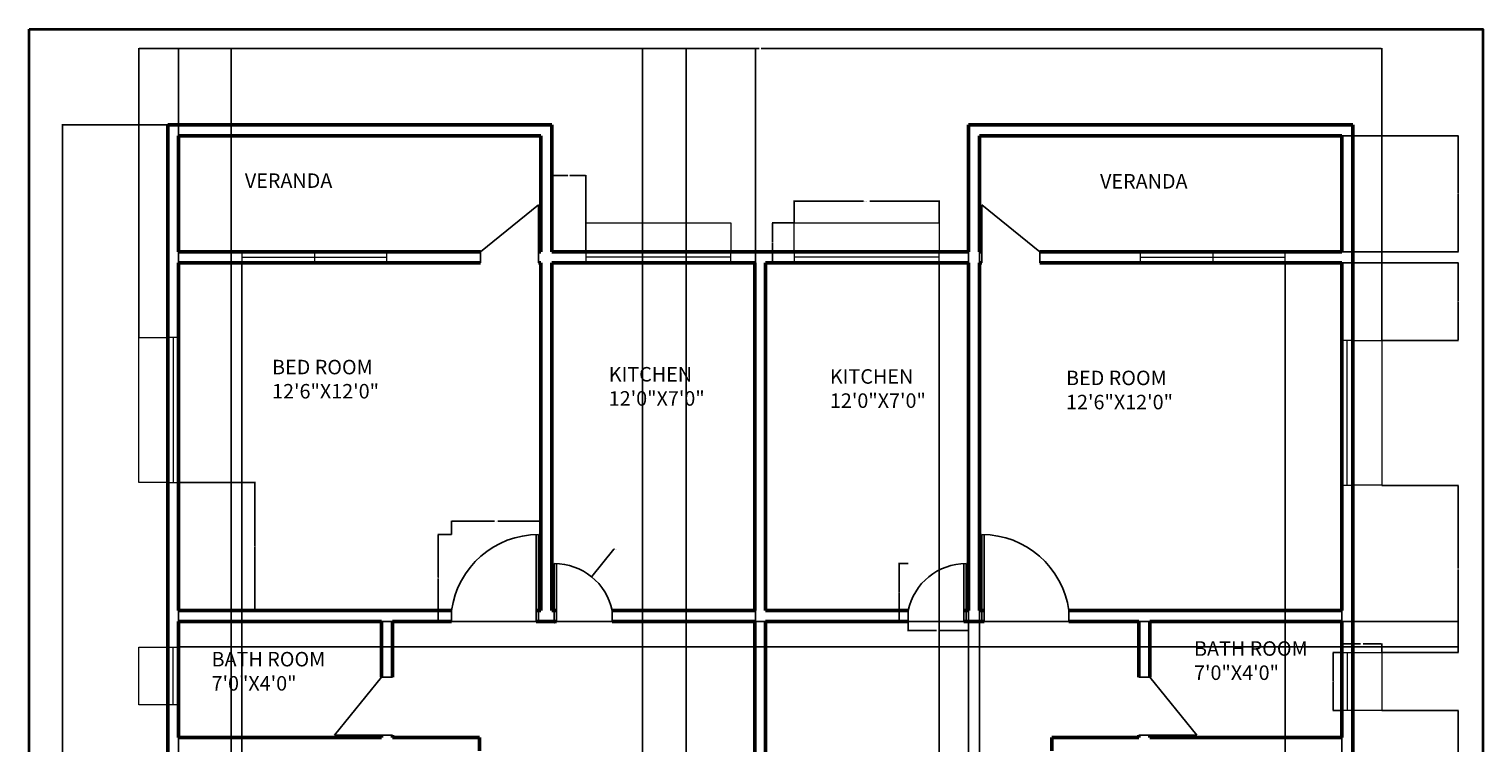
# Model space of a CAD drawing. Units: inches. Extents: x 2412 to 3014, y 10657 to 11360.
# Tile 3 of 3: x 2412 to 3014, y 11065 to 11360. Entities that reach past the tile are written whole.
import ezdxf

# ---------------------------------------------------------------- set-up
doc = ezdxf.new("R2010")
doc.units = ezdxf.units.IN
doc.header["$MEASUREMENT"] = 0
for name, color, linetype, lineweight in [('A-ANNO-DIMS', 2, 'Continuous', 18), ('A-ANNO-TTLB', 7, 'Continuous', 35), ('A-AREA-IDEN', 7, 'Continuous', 18), ('A-DOOR', 22, 'Continuous', 25), ('A-GLAZ', 160, 'Continuous', 18), ('A-WALL', 142, 'Continuous', 50)]:
    doc.layers.add(name, color=color, linetype=linetype, lineweight=lineweight)
doc.styles.get("Standard").update_dxf_attribs({"font": 'arial.ttf'})
doc.dimstyles.get("Standard").update_dxf_attribs({"dimtxt": 0.18, "dimasz": 0.18, "dimexe": 0.18, "dimexo": 0.0625, "dimgap": 0.09, "dimtad": 0, "dimtih": 1, "dimtoh": 1, "dimdec": 4, "dimzin": 0, "dimdsep": 46, "dimtxsty": 'Standard', "dimcen": 0.09, "dimadec": 0, "dimazin": 0, "dimtfac": 1, "dimtdec": 4, "dimtofl": 0, "dimtmove": 0, "dimatfit": 3, "dimfxl": 1, "dimtolj": 1, "dimtzin": 0, "dimarcsym": 0})

# ---------------------------------------------------------------- blocks, each defined once
blk = doc.blocks.new('WIN-60IN-PROJECTING-SILL')
for p, q in [((0, 0), (0, 12)), ((0, 12), (60, 12)), ((60, 12), (60, 0)), ((0, 0), (0, -4.5)), ((60, 0), (0, 0)), ((60, -4.5), (60, 0)), ((60, -2.25), (0, -2.25)), ((0, -4.5), (60, -4.5))]:
    blk.add_line(p, q)
blk = doc.blocks.new('VENT-24IN-PROJECTING-SILL')
for p, q in [((0, 0), (4.5, 0)), ((0, -24), (0, 0)), ((2.25, 0), (2.25, -24)), ((4.5, 0), (4.5, -24)), ((4.5, 0), (16.5, 0)), ((16.5, 0), (16.5, -24)), ((4.5, -24), (0, -24)), ((16.5, -24), (4.5, -24))]:
    blk.add_line(p, q)
blk = doc.blocks.new('WIN-60IN-DIVIDED')
for p, q in [((0, 0), (0, -4.5)), ((60, 0), (0, 0)), ((30, 0), (30, -4.5)), ((60, -4.5), (60, 0)), ((0, -2.25), (60, -2.25)), ((0, -4.5), (60, -4.5))]:
    blk.add_line(p, q)
blk = doc.blocks.new('DOOR-36IN-ARC')
for p, q in [((-1, 36), (-1, 0)), ((0, 0), (0, 36)), ((0, 36), (0, 0)), ((-36, 0), (-36, 4.5)), ((0, 0), (-1, 0)), ((1, 0), (0, 0))]:
    blk.add_line(p, q)
blk.add_arc((0, -0.32), 36.32, 90, 172.37185)
blk = doc.blocks.new('DOOR-24IN-ARC')
for p, q in [((0, 0), (0, 24)), ((0, 24), (0, 0)), ((1, 24), (1, 0)), ((-1, 0), (0, 0)), ((0, 0), (1, 0)), ((24, 0), (24, 4.5))]:
    blk.add_line(p, q)
blk.add_arc((0, -0.52), 24.52, 11.81228, 90)
blk = doc.blocks.new('DOOR-24IN-DIAGONAL')
for p, q in [((0, 24), (-24, 4.5)), ((0, 0), (0, 24)), ((0, 24), (0, 0)), ((-24, 0), (-24, 4.5)), ((1, 0), (0, 0))]:
    blk.add_line(p, q)
blk = doc.blocks.new('*D8')
at = {"layer": 'A-ANNO-DIMS', "color": 0, "lineweight": -2, "transparency": 16777216}
for p, q in [((2729.19, 11280.34), (2729.19, 11289.46)), ((2789.19, 11280.34), (2789.19, 11289.46)), ((2729.37, 11289.28), (2757.85, 11289.28)), ((2789.01, 11289.28), (2760.54, 11289.28))]:
    blk.add_line(p, q, dxfattribs=at)
at = {"layer": 'A-ANNO-DIMS', "color": 0, "transparency": 16777216}
for points in [[(2729.37, 11289.31), (2729.37, 11289.25), (2729.19, 11289.28)], [(2789.01, 11289.31), (2789.01, 11289.25), (2789.19, 11289.28)]]:
    blk.add_solid(points, dxfattribs=at)
at = {"layer": 'Defpoints', "color": 0, "transparency": 16777216}
for p in [(2789.19, 11289.28), (2729.19, 11280.28), (2789.19, 11280.28)]:
    blk.add_point(p, dxfattribs=at)
at = {"layer": 'A-ANNO-DIMS', "color": 0, "transparency": 16777216, "insert": (2759.19, 11289.28), "char_height": 0.18, "attachment_point": 5}
blk.add_mtext('\\A1;WINDOW W1 60 TYP.', dxfattribs=at)
blk = doc.blocks.new('*D9')
at = {"layer": 'A-ANNO-DIMS', "color": 0, "lineweight": -2, "transparency": 16777216}
for p, q in [((2729.13, 11280.28), (2720.01, 11280.28)), ((2720.19, 11280.1), (2720.19, 11272.21)), ((2720.19, 11263.96), (2720.19, 11271.85)), ((2729.13, 11263.78), (2720.01, 11263.78))]:
    blk.add_line(p, q, dxfattribs=at)
at = {"layer": 'A-ANNO-DIMS', "color": 0, "transparency": 16777216}
for points in [[(2720.16, 11280.1), (2720.22, 11280.1), (2720.19, 11280.28)], [(2720.16, 11263.96), (2720.22, 11263.96), (2720.19, 11263.78)]]:
    blk.add_solid(points, dxfattribs=at)
at = {"layer": 'Defpoints', "color": 0, "transparency": 16777216}
for p in [(2720.19, 11280.28), (2729.19, 11280.28), (2729.19, 11263.78)]:
    blk.add_point(p, dxfattribs=at)
at = {"layer": 'A-ANNO-DIMS', "color": 0, "transparency": 16777216, "insert": (2720.19, 11272.03), "char_height": 0.18, "attachment_point": 5}
blk.add_mtext('\\A1;17 TYP.', dxfattribs=at)
blk = doc.blocks.new('*D12')
at = {"layer": 'A-ANNO-DIMS', "color": 0, "lineweight": -2, "transparency": 16777216}
for p, q in [((2955.8, 11102.46), (2952.08, 11102.46)), ((2952.26, 11102.28), (2952.26, 11090.64)), ((2952.26, 11078.64), (2952.26, 11090.28)), ((2955.8, 11078.46), (2952.08, 11078.46))]:
    blk.add_line(p, q, dxfattribs=at)
at = {"layer": 'A-ANNO-DIMS', "color": 0, "transparency": 16777216}
for points in [[(2952.23, 11102.28), (2952.29, 11102.28), (2952.26, 11102.46)], [(2952.23, 11078.64), (2952.29, 11078.64), (2952.26, 11078.46)]]:
    blk.add_solid(points, dxfattribs=at)
at = {"layer": 'Defpoints', "color": 0, "transparency": 16777216}
for p in [(2952.26, 11102.46), (2955.86, 11102.46), (2955.86, 11078.46)]:
    blk.add_point(p, dxfattribs=at)
at = {"layer": 'A-ANNO-DIMS', "color": 0, "transparency": 16777216, "insert": (2952.26, 11090.46), "char_height": 0.18, "attachment_point": 5}
blk.add_mtext('\\A1;VENT 24 TYP.', dxfattribs=at)
blk = doc.blocks.new('*D13')
at = {"layer": 'A-ANNO-DIMS', "color": 0, "lineweight": -2, "transparency": 16777216}
for p, q in [((2955.86, 11102.52), (2955.86, 11106.24)), ((2956.04, 11106.06), (2963.59, 11106.06)), ((2972.18, 11106.06), (2964.63, 11106.06)), ((2972.36, 11102.52), (2972.36, 11106.24))]:
    blk.add_line(p, q, dxfattribs=at)
at = {"layer": 'A-ANNO-DIMS', "color": 0, "transparency": 16777216}
for points in [[(2956.04, 11106.09), (2956.04, 11106.03), (2955.86, 11106.06)], [(2972.18, 11106.09), (2972.18, 11106.03), (2972.36, 11106.06)]]:
    blk.add_solid(points, dxfattribs=at)
at = {"layer": 'Defpoints', "color": 0, "transparency": 16777216}
for p in [(2972.36, 11106.06), (2955.86, 11102.46), (2972.36, 11102.46)]:
    blk.add_point(p, dxfattribs=at)
at = {"layer": 'A-ANNO-DIMS', "color": 0, "transparency": 16777216, "insert": (2964.11, 11106.06), "char_height": 0.18, "attachment_point": 5}
blk.add_mtext('\\A1;17 TYP.', dxfattribs=at)
blk = doc.blocks.new('*D14')
at = {"layer": 'A-ANNO-DIMS', "color": 0, "lineweight": -2, "transparency": 16777216}
for p, q in [((2587.36, 11151.34), (2587.36, 11157.01)), ((2624.36, 11151.34), (2624.36, 11157.01)), ((2587.54, 11156.83), (2605.14, 11156.83)), ((2624.18, 11156.83), (2606.58, 11156.83))]:
    blk.add_line(p, q, dxfattribs=at)
at = {"layer": 'A-ANNO-DIMS', "color": 0, "transparency": 16777216}
for points in [[(2587.54, 11156.86), (2587.54, 11156.8), (2587.36, 11156.83)], [(2624.18, 11156.86), (2624.18, 11156.8), (2624.36, 11156.83)]]:
    blk.add_solid(points, dxfattribs=at)
at = {"layer": 'Defpoints', "color": 0, "transparency": 16777216}
for p in [(2587.36, 11151.28), (2624.36, 11156.83), (2624.36, 11151.28)]:
    blk.add_point(p, dxfattribs=at)
at = {"layer": 'A-ANNO-DIMS', "color": 0, "transparency": 16777216, "insert": (2605.86, 11156.83), "char_height": 0.18, "attachment_point": 5}
blk.add_mtext('\\A1;D1 37 TYP.', dxfattribs=at)
blk = doc.blocks.new('*D15')
at = {"layer": 'A-ANNO-DIMS', "color": 0, "lineweight": -2, "transparency": 16777216}
for p, q in [((2587.3, 11151.28), (2581.63, 11151.28)), ((2581.81, 11151.1), (2581.81, 11133.46)), ((2581.81, 11115.46), (2581.81, 11133.1)), ((2587.3, 11115.28), (2581.63, 11115.28))]:
    blk.add_line(p, q, dxfattribs=at)
at = {"layer": 'A-ANNO-DIMS', "color": 0, "transparency": 16777216}
for points in [[(2581.78, 11151.1), (2581.84, 11151.1), (2581.81, 11151.28)], [(2581.78, 11115.46), (2581.84, 11115.46), (2581.81, 11115.28)]]:
    blk.add_solid(points, dxfattribs=at)
at = {"layer": 'Defpoints', "color": 0, "transparency": 16777216}
for p in [(2581.81, 11151.28), (2587.36, 11151.28), (2587.36, 11115.28)]:
    blk.add_point(p, dxfattribs=at)
at = {"layer": 'A-ANNO-DIMS', "color": 0, "transparency": 16777216, "insert": (2581.81, 11133.28), "char_height": 0.18, "attachment_point": 5}
blk.add_mtext('\\A1;36 TYP.', dxfattribs=at)
blk = doc.blocks.new('*D16')
at = {"layer": 'A-ANNO-DIMS', "color": 0, "lineweight": -2, "transparency": 16777216}
for p, q in [((2776.36, 11115.22), (2776.36, 11111.35)), ((2801.36, 11115.22), (2801.36, 11111.35)), ((2776.54, 11111.53), (2788.14, 11111.53)), ((2801.18, 11111.53), (2789.58, 11111.53))]:
    blk.add_line(p, q, dxfattribs=at)
at = {"layer": 'A-ANNO-DIMS', "color": 0, "transparency": 16777216}
for points in [[(2776.54, 11111.56), (2776.54, 11111.5), (2776.36, 11111.53)], [(2801.18, 11111.56), (2801.18, 11111.5), (2801.36, 11111.53)]]:
    blk.add_solid(points, dxfattribs=at)
at = {"layer": 'Defpoints', "color": 0, "transparency": 16777216}
for p in [(2776.36, 11115.28), (2801.36, 11115.28), (2776.36, 11111.53)]:
    blk.add_point(p, dxfattribs=at)
at = {"layer": 'A-ANNO-DIMS', "color": 0, "transparency": 16777216, "insert": (2788.86, 11111.53), "char_height": 0.18, "attachment_point": 5}
blk.add_mtext('\\A1;D2 25 TYP.', dxfattribs=at)
blk = doc.blocks.new('*D17')
at = {"layer": 'A-ANNO-DIMS', "color": 0, "lineweight": -2, "transparency": 16777216}
for p, q in [((2776.3, 11139.28), (2772.43, 11139.28)), ((2772.61, 11139.1), (2772.61, 11127.46)), ((2772.61, 11115.46), (2772.61, 11127.1)), ((2776.3, 11115.28), (2772.43, 11115.28))]:
    blk.add_line(p, q, dxfattribs=at)
at = {"layer": 'A-ANNO-DIMS', "color": 0, "transparency": 16777216}
for points in [[(2772.58, 11139.1), (2772.64, 11139.1), (2772.61, 11139.28)], [(2772.58, 11115.46), (2772.64, 11115.46), (2772.61, 11115.28)]]:
    blk.add_solid(points, dxfattribs=at)
at = {"layer": 'Defpoints', "color": 0, "transparency": 16777216}
for p in [(2772.61, 11139.28), (2776.36, 11139.28), (2776.36, 11115.28)]:
    blk.add_point(p, dxfattribs=at)
at = {"layer": 'A-ANNO-DIMS', "color": 0, "transparency": 16777216, "insert": (2772.61, 11127.28), "char_height": 0.18, "attachment_point": 5}
blk.add_mtext('\\A1;24 TYP.', dxfattribs=at)
blk = doc.blocks.new('*D22')
at = {"layer": 'A-ANNO-DIMS', "color": 0, "lineweight": -2, "transparency": 16777216}
for p, q in [((2457.86, 11232.92), (2457.86, 11352.57)), ((2458.04, 11352.39), (2714.72, 11352.39)), ((2972.18, 11352.39), (2715.51, 11352.39)), ((2972.36, 11231.71), (2972.36, 11352.57))]:
    blk.add_line(p, q, dxfattribs=at)
at = {"layer": 'A-ANNO-DIMS', "color": 0, "transparency": 16777216}
for points in [[(2458.04, 11352.42), (2458.04, 11352.36), (2457.86, 11352.39)], [(2972.18, 11352.42), (2972.18, 11352.36), (2972.36, 11352.39)]]:
    blk.add_solid(points, dxfattribs=at)
at = {"layer": 'Defpoints', "color": 0, "transparency": 16777216}
for p in [(2972.36, 11352.39), (2457.86, 11232.86), (2972.36, 11231.64)]:
    blk.add_point(p, dxfattribs=at)
at = {"layer": 'A-ANNO-DIMS', "color": 0, "transparency": 16777216, "insert": (2715.11, 11352.39), "char_height": 0.18, "attachment_point": 5}
blk.add_mtext('\\A1;514.5', dxfattribs=at)
blk = doc.blocks.new('*D23')
at = {"layer": 'A-ANNO-DIMS', "color": 0, "lineweight": -2, "transparency": 16777216}
for p, q in [((2469.8, 11320.78), (2426.08, 11320.78)), ((2426.26, 11320.6), (2426.26, 11005.21)), ((2426.26, 10689.46), (2426.26, 11004.85)), ((2684.42, 10689.28), (2426.08, 10689.28))]:
    blk.add_line(p, q, dxfattribs=at)
at = {"layer": 'A-ANNO-DIMS', "color": 0, "transparency": 16777216}
for points in [[(2426.23, 11320.6), (2426.29, 11320.6), (2426.26, 11320.78)], [(2426.23, 10689.46), (2426.29, 10689.46), (2426.26, 10689.28)]]:
    blk.add_solid(points, dxfattribs=at)
at = {"layer": 'Defpoints', "color": 0, "transparency": 16777216}
for p in [(2426.26, 11320.78), (2469.86, 11320.78), (2684.48, 10689.28)]:
    blk.add_point(p, dxfattribs=at)
at = {"layer": 'A-ANNO-DIMS', "color": 0, "transparency": 16777216, "insert": (2426.26, 11005.03), "char_height": 0.18, "attachment_point": 5}
blk.add_mtext('\\A1;631.5', dxfattribs=at)
blk = doc.blocks.new('*D29')
at = {"layer": 'A-ANNO-DIMS', "color": 0, "lineweight": -2, "transparency": 16777216}
for p, q in [((2801.36, 11320.72), (2801.36, 10657.5)), ((2805.86, 11316.22), (2805.86, 10657.5)), ((2801.54, 10657.68), (2803.35, 10657.68)), ((2805.68, 10657.68), (2803.87, 10657.68))]:
    blk.add_line(p, q, dxfattribs=at)
at = {"layer": 'A-ANNO-DIMS', "color": 0, "transparency": 16777216}
for points in [[(2801.54, 10657.71), (2801.54, 10657.65), (2801.36, 10657.68)], [(2805.68, 10657.71), (2805.68, 10657.65), (2805.86, 10657.68)]]:
    blk.add_solid(points, dxfattribs=at)
at = {"layer": 'Defpoints', "color": 0, "transparency": 16777216}
for p in [(2801.36, 11320.78), (2805.86, 11316.28), (2805.86, 10657.68)]:
    blk.add_point(p, dxfattribs=at)
at = {"layer": 'A-ANNO-DIMS', "color": 0, "transparency": 16777216, "insert": (2803.61, 10657.68), "char_height": 0.18, "attachment_point": 5}
blk.add_mtext('\\A1;4.5', dxfattribs=at)
blk = doc.blocks.new('*D30')
at = {"layer": 'A-ANNO-DIMS', "color": 0, "lineweight": -2, "transparency": 16777216}
for p, q in [((2666.36, 10859.68), (2666.36, 11352.57)), ((2666.54, 11352.39), (2689.34, 11352.39)), ((2712.93, 11352.39), (2690.13, 11352.39)), ((2713.11, 10859.68), (2713.11, 11352.57))]:
    blk.add_line(p, q, dxfattribs=at)
at = {"layer": 'A-ANNO-DIMS', "color": 0, "transparency": 16777216}
for points in [[(2666.54, 11352.42), (2666.54, 11352.36), (2666.36, 11352.39)], [(2712.93, 11352.42), (2712.93, 11352.36), (2713.11, 11352.39)]]:
    blk.add_solid(points, dxfattribs=at)
at = {"layer": 'Defpoints', "color": 0, "transparency": 16777216}
for p in [(2713.11, 11352.39), (2666.36, 10859.62), (2713.11, 10859.62)]:
    blk.add_point(p, dxfattribs=at)
at = {"layer": 'A-ANNO-DIMS', "color": 0, "transparency": 16777216, "insert": (2689.74, 11352.39), "char_height": 0.18, "attachment_point": 5}
blk.add_mtext('\\A1;46.75', dxfattribs=at)
blk = doc.blocks.new('*D36')
at = {"layer": 'A-ANNO-DIMS', "color": 0, "lineweight": -2, "transparency": 16777216}
for p, q in [((2972.42, 11078.46), (3004.15, 11078.46)), ((3003.97, 11078.28), (3003.97, 11045.74)), ((3003.97, 11012.83), (3003.97, 11045.37)), ((2972.42, 11012.65), (3004.15, 11012.65))]:
    blk.add_line(p, q, dxfattribs=at)
at = {"layer": 'A-ANNO-DIMS', "color": 0, "transparency": 16777216}
for points in [[(3003.94, 11078.28), (3004, 11078.28), (3003.97, 11078.46)], [(3003.94, 11012.83), (3004, 11012.83), (3003.97, 11012.65)]]:
    blk.add_solid(points, dxfattribs=at)
at = {"layer": 'Defpoints', "color": 0, "transparency": 16777216}
for p in [(2972.36, 11078.46), (3003.97, 11078.46), (2972.36, 11012.65)]:
    blk.add_point(p, dxfattribs=at)
at = {"layer": 'A-ANNO-DIMS', "color": 0, "transparency": 16777216, "insert": (3003.97, 11045.55), "char_height": 0.18, "attachment_point": 5}
blk.add_mtext('\\A1;65.82', dxfattribs=at)
blk = doc.blocks.new('*D37')
at = {"layer": 'A-ANNO-DIMS', "color": 0, "lineweight": -2, "transparency": 16777216}
for p, q in [((2972.42, 11171.64), (3004.15, 11171.64)), ((3003.97, 11171.46), (3003.97, 11137.23)), ((3003.97, 11102.64), (3003.97, 11136.87)), ((2972.42, 11102.46), (3004.15, 11102.46))]:
    blk.add_line(p, q, dxfattribs=at)
at = {"layer": 'A-ANNO-DIMS', "color": 0, "transparency": 16777216}
for points in [[(3003.94, 11171.46), (3004, 11171.46), (3003.97, 11171.64)], [(3003.94, 11102.64), (3004, 11102.64), (3003.97, 11102.46)]]:
    blk.add_solid(points, dxfattribs=at)
at = {"layer": 'Defpoints', "color": 0, "transparency": 16777216}
for p in [(2972.36, 11171.64), (3003.97, 11171.64), (2972.36, 11102.46)]:
    blk.add_point(p, dxfattribs=at)
at = {"layer": 'A-ANNO-DIMS', "color": 0, "transparency": 16777216, "insert": (3003.97, 11137.05), "char_height": 0.18, "attachment_point": 5}
blk.add_mtext('\\A1;69.18', dxfattribs=at)
blk = doc.blocks.new('*D38')
at = {"layer": 'A-ANNO-DIMS', "color": 0, "lineweight": -2, "transparency": 16777216}
for p, q in [((2955.92, 11263.78), (3004.15, 11263.78)), ((3003.97, 11263.6), (3003.97, 11247.89)), ((3003.97, 11231.82), (3003.97, 11247.53)), ((2972.42, 11231.64), (3004.15, 11231.64))]:
    blk.add_line(p, q, dxfattribs=at)
at = {"layer": 'A-ANNO-DIMS', "color": 0, "transparency": 16777216}
for points in [[(3003.94, 11263.6), (3004, 11263.6), (3003.97, 11263.78)], [(3003.94, 11231.82), (3004, 11231.82), (3003.97, 11231.64)]]:
    blk.add_solid(points, dxfattribs=at)
at = {"layer": 'Defpoints', "color": 0, "transparency": 16777216}
for p in [(2955.86, 11263.78), (3003.97, 11263.78), (2972.36, 11231.64)]:
    blk.add_point(p, dxfattribs=at)
at = {"layer": 'A-ANNO-DIMS', "color": 0, "transparency": 16777216, "insert": (3003.97, 11247.71), "char_height": 0.18, "attachment_point": 5}
blk.add_mtext('\\A1;32.14', dxfattribs=at)
blk = doc.blocks.new('*D39')
at = {"layer": 'A-ANNO-DIMS', "color": 0, "lineweight": -2, "transparency": 16777216}
for p, q in [((2955.92, 11316.28), (3004.15, 11316.28)), ((3003.97, 11316.1), (3003.97, 11292.46)), ((3003.97, 11268.46), (3003.97, 11292.1)), ((2955.92, 11268.28), (3004.15, 11268.28))]:
    blk.add_line(p, q, dxfattribs=at)
at = {"layer": 'A-ANNO-DIMS', "color": 0, "transparency": 16777216}
for points in [[(3003.94, 11316.1), (3004, 11316.1), (3003.97, 11316.28)], [(3003.94, 11268.46), (3004, 11268.46), (3003.97, 11268.28)]]:
    blk.add_solid(points, dxfattribs=at)
at = {"layer": 'Defpoints', "color": 0, "transparency": 16777216}
for p in [(2955.86, 11316.28), (3003.97, 11316.28), (2955.86, 11268.28)]:
    blk.add_point(p, dxfattribs=at)
at = {"layer": 'A-ANNO-DIMS', "color": 0, "transparency": 16777216, "insert": (3003.97, 11292.28), "char_height": 0.18, "attachment_point": 5}
blk.add_mtext('\\A1;48', dxfattribs=at)
blk = doc.blocks.new('*D40')
at = {"layer": 'A-ANNO-DIMS', "color": 0, "lineweight": -2, "transparency": 16777216}
for p, q in [((2474.36, 11263.72), (2474.36, 10657.5)), ((2500.62, 11263.72), (2500.62, 10657.5)), ((2474.54, 10657.68), (2487.1, 10657.68)), ((2500.44, 10657.68), (2487.89, 10657.68))]:
    blk.add_line(p, q, dxfattribs=at)
at = {"layer": 'A-ANNO-DIMS', "color": 0, "transparency": 16777216}
for points in [[(2474.54, 10657.71), (2474.54, 10657.65), (2474.36, 10657.68)], [(2500.44, 10657.71), (2500.44, 10657.65), (2500.62, 10657.68)]]:
    blk.add_solid(points, dxfattribs=at)
at = {"layer": 'Defpoints', "color": 0, "transparency": 16777216}
for p in [(2474.36, 11263.78), (2500.62, 11263.78), (2500.62, 10657.68)]:
    blk.add_point(p, dxfattribs=at)
at = {"layer": 'A-ANNO-DIMS', "color": 0, "transparency": 16777216, "insert": (2487.49, 10657.68), "char_height": 0.18, "attachment_point": 5}
blk.add_mtext('\\A1;26.26', dxfattribs=at)
blk = doc.blocks.new('*D41')
at = {"layer": 'A-ANNO-DIMS', "color": 0, "lineweight": -2, "transparency": 16777216}
for p, q in [((2628.86, 11268.34), (2628.86, 11300.07)), ((2629.04, 11299.89), (2635.52, 11299.89)), ((2642.77, 11299.89), (2636.29, 11299.89)), ((2642.95, 11268.34), (2642.95, 11300.07))]:
    blk.add_line(p, q, dxfattribs=at)
at = {"layer": 'A-ANNO-DIMS', "color": 0, "transparency": 16777216}
for points in [[(2629.04, 11299.92), (2629.04, 11299.86), (2628.86, 11299.89)], [(2642.77, 11299.92), (2642.77, 11299.86), (2642.95, 11299.89)]]:
    blk.add_solid(points, dxfattribs=at)
at = {"layer": 'Defpoints', "color": 0, "transparency": 16777216}
for p in [(2642.95, 11299.89), (2628.86, 11268.28), (2642.95, 11268.28)]:
    blk.add_point(p, dxfattribs=at)
at = {"layer": 'A-ANNO-DIMS', "color": 0, "transparency": 16777216, "insert": (2635.91, 11299.89), "char_height": 0.18, "attachment_point": 5}
blk.add_mtext('\\A1;14.09', dxfattribs=at)
blk = doc.blocks.new('*D42')
at = {"layer": 'A-ANNO-DIMS', "color": 0, "lineweight": -2, "transparency": 16777216}
for p, q in [((2474.36, 10758.34), (2474.36, 11352.57)), ((2474.54, 11352.39), (2484.85, 11352.39)), ((2495.94, 11352.39), (2485.64, 11352.39)), ((2496.12, 10758.34), (2496.12, 11352.57))]:
    blk.add_line(p, q, dxfattribs=at)
at = {"layer": 'A-ANNO-DIMS', "color": 0, "transparency": 16777216}
for points in [[(2474.54, 11352.42), (2474.54, 11352.36), (2474.36, 11352.39)], [(2495.94, 11352.42), (2495.94, 11352.36), (2496.12, 11352.39)]]:
    blk.add_solid(points, dxfattribs=at)
at = {"layer": 'Defpoints', "color": 0, "transparency": 16777216}
for p in [(2496.12, 11352.39), (2474.36, 10758.28), (2496.12, 10758.28)]:
    blk.add_point(p, dxfattribs=at)
at = {"layer": 'A-ANNO-DIMS', "color": 0, "transparency": 16777216, "insert": (2485.24, 11352.39), "char_height": 0.18, "attachment_point": 5}
blk.add_mtext('\\A1;21.76', dxfattribs=at)
blk = doc.blocks.new('*D43')
at = {"layer": 'A-ANNO-DIMS', "color": 0, "lineweight": -2, "transparency": 16777216}
for p, q in [((2474.42, 11172.86), (2506.15, 11172.86)), ((2505.97, 11172.68), (2505.97, 11146.5)), ((2505.97, 11119.96), (2505.97, 11146.14)), ((2474.42, 11119.78), (2506.15, 11119.78))]:
    blk.add_line(p, q, dxfattribs=at)
at = {"layer": 'A-ANNO-DIMS', "color": 0, "transparency": 16777216}
for points in [[(2505.94, 11172.68), (2506, 11172.68), (2505.97, 11172.86)], [(2505.94, 11119.96), (2506, 11119.96), (2505.97, 11119.78)]]:
    blk.add_solid(points, dxfattribs=at)
at = {"layer": 'Defpoints', "color": 0, "transparency": 16777216}
for p in [(2474.36, 11172.86), (2474.36, 11119.78), (2505.97, 11119.78)]:
    blk.add_point(p, dxfattribs=at)
at = {"layer": 'A-ANNO-DIMS', "color": 0, "transparency": 16777216, "insert": (2505.97, 11146.32), "char_height": 0.18, "attachment_point": 5}
blk.add_mtext('\\A1;53.08', dxfattribs=at)
blk = doc.blocks.new('*D44')
at = {"layer": 'A-ANNO-DIMS', "color": 0, "lineweight": -2, "transparency": 16777216}
for p, q in [((2474.42, 11115.28), (3004.15, 11115.28)), ((3003.97, 11115.1), (3003.97, 11110.19)), ((3003.97, 11104.91), (3003.97, 11109.82)), ((2474.42, 11104.73), (3004.15, 11104.73))]:
    blk.add_line(p, q, dxfattribs=at)
at = {"layer": 'A-ANNO-DIMS', "color": 0, "transparency": 16777216}
for points in [[(3003.94, 11115.1), (3004, 11115.1), (3003.97, 11115.28)], [(3003.94, 11104.91), (3004, 11104.91), (3003.97, 11104.73)]]:
    blk.add_solid(points, dxfattribs=at)
at = {"layer": 'Defpoints', "color": 0, "transparency": 16777216}
for p in [(2474.36, 11115.28), (3003.97, 11115.28), (2474.36, 11104.73)]:
    blk.add_point(p, dxfattribs=at)
at = {"layer": 'A-ANNO-DIMS', "color": 0, "transparency": 16777216, "insert": (3003.97, 11110), "char_height": 0.18, "attachment_point": 5}
blk.add_mtext('\\A1;10.553', dxfattribs=at)
blk = doc.blocks.new('*D47')
at = {"layer": 'A-ANNO-DIMS', "color": 0, "lineweight": -2, "transparency": 16777216}
for p, q in [((2932.41, 11263.72), (2932.41, 10657.5)), ((2955.86, 11263.72), (2955.86, 10657.5)), ((2932.59, 10657.68), (2943.67, 10657.68)), ((2955.68, 10657.68), (2944.6, 10657.68))]:
    blk.add_line(p, q, dxfattribs=at)
at = {"layer": 'A-ANNO-DIMS', "color": 0, "transparency": 16777216}
for points in [[(2932.59, 10657.71), (2932.59, 10657.65), (2932.41, 10657.68)], [(2955.68, 10657.71), (2955.68, 10657.65), (2955.86, 10657.68)]]:
    blk.add_solid(points, dxfattribs=at)
at = {"layer": 'Defpoints', "color": 0, "transparency": 16777216}
for p in [(2932.41, 11263.78), (2955.86, 11263.78), (2955.86, 10657.68)]:
    blk.add_point(p, dxfattribs=at)
at = {"layer": 'A-ANNO-DIMS', "color": 0, "transparency": 16777216, "insert": (2944.13, 10657.68), "char_height": 0.18, "attachment_point": 5}
blk.add_mtext('\\A1;23.453', dxfattribs=at)
blk = doc.blocks.new('*D48')
at = {"layer": 'A-ANNO-DIMS', "color": 0, "lineweight": -2, "transparency": 16777216}
for p, q in [((2789.19, 11263.72), (2789.19, 10657.5)), ((2801.36, 11263.72), (2801.36, 10657.5)), ((2789.37, 10657.68), (2794.82, 10657.68)), ((2801.18, 10657.68), (2795.73, 10657.68))]:
    blk.add_line(p, q, dxfattribs=at)
at = {"layer": 'A-ANNO-DIMS', "color": 0, "transparency": 16777216}
for points in [[(2789.37, 10657.71), (2789.37, 10657.65), (2789.19, 10657.68)], [(2801.18, 10657.71), (2801.18, 10657.65), (2801.36, 10657.68)]]:
    blk.add_solid(points, dxfattribs=at)
at = {"layer": 'Defpoints', "color": 0, "transparency": 16777216}
for p in [(2789.19, 11263.78), (2801.36, 11263.78), (2801.36, 10657.68)]:
    blk.add_point(p, dxfattribs=at)
at = {"layer": 'A-ANNO-DIMS', "color": 0, "transparency": 16777216, "insert": (2795.28, 10657.68), "char_height": 0.18, "attachment_point": 5}
blk.add_mtext('\\A1;12.166', dxfattribs=at)
blk = doc.blocks.new('*D50')
at = {"layer": 'A-ANNO-DIMS', "color": 0, "lineweight": -2, "transparency": 16777216}
for p, q in [((2666.36, 10705.84), (2666.36, 11352.57)), ((2666.54, 11352.39), (2674.96, 11352.39)), ((2684.3, 11352.39), (2675.87, 11352.39)), ((2684.48, 10705.84), (2684.48, 11352.57))]:
    blk.add_line(p, q, dxfattribs=at)
at = {"layer": 'A-ANNO-DIMS', "color": 0, "transparency": 16777216}
for points in [[(2666.54, 11352.42), (2666.54, 11352.36), (2666.36, 11352.39)], [(2684.3, 11352.42), (2684.3, 11352.36), (2684.48, 11352.39)]]:
    blk.add_solid(points, dxfattribs=at)
at = {"layer": 'Defpoints', "color": 0, "transparency": 16777216}
for p in [(2684.48, 11352.39), (2666.36, 10705.78), (2684.48, 10705.78)]:
    blk.add_point(p, dxfattribs=at)
at = {"layer": 'A-ANNO-DIMS', "color": 0, "transparency": 16777216, "insert": (2675.42, 11352.39), "char_height": 0.18, "attachment_point": 5}
blk.add_mtext('\\A1;18.116', dxfattribs=at)
blk = doc.blocks.new('*D52')
at = {"layer": 'A-ANNO-DIMS', "color": 0, "lineweight": -2, "transparency": 16777216}
for p, q in [((2654.6, 11145.21), (2645.44, 11133.93)), ((2654.78, 11145.21), (2654.6, 11145.21)), ((2629.86, 11114.67), (2629.86, 11114.85)), ((2629.77, 11114.76), (2629.95, 11114.76))]:
    blk.add_line(p, q, dxfattribs=at)
at = {"layer": 'A-ANNO-DIMS', "color": 0, "transparency": 16777216}
blk.add_solid([(2645.41, 11133.95), (2645.46, 11133.91), (2645.32, 11133.79)], dxfattribs=at)
at = {"layer": 'Defpoints', "color": 0, "transparency": 16777216}
for p in [(2645.32, 11133.79), (2629.86, 11114.76)]:
    blk.add_point(p, dxfattribs=at)
at = {"layer": 'A-ANNO-DIMS', "color": 0, "transparency": 16777216, "insert": (2655.45, 11145.21), "char_height": 0.18, "attachment_point": 5}
blk.add_mtext('\\A1;2X R24.52', dxfattribs=at)

msp = doc.modelspace()

# ---------------------------------------------------------------- linework, layer by layer
at = {"layer": 'A-ANNO-TTLB'}
msp.add_lwpolyline([(2412.4885, 11360.4742), (3014.2671, 11360.4742), (3014.2671, 10657.3977), (2412.4885, 10657.3977)], close=True, dxfattribs=at)
at = {"layer": 'A-WALL'}
for p, q in [((2469.8613, 11320.7803), (2469.8613, 10701.2803)), ((2469.8613, 11320.7803), (2628.8613, 11320.7803)), ((2628.8613, 11320.7803), (2628.8613, 11268.2803)), ((2801.3613, 11320.7803), (2801.3613, 11268.2803)), ((2801.3613, 11320.7803), (2960.3613, 11320.7803)), ((2960.3613, 11320.7803), (2960.3613, 10701.2803)), ((2474.3613, 11316.2803), (2474.3613, 11268.2803)), ((2474.3613, 11316.2803), (2624.3613, 11316.2803)), ((2624.3613, 11316.2803), (2624.3613, 11268.2803)), ((2805.8613, 11316.2803), (2805.8613, 11268.2803)), ((2805.8613, 11316.2803), (2955.8613, 11316.2803)), ((2955.8613, 11316.2803), (2955.8613, 11268.2803)), ((2474.3613, 11268.2803), (2599.3613, 11268.2803)), ((2623.3613, 11268.2803), (2624.3613, 11268.2803)), ((2628.8613, 11268.2803), (2801.3613, 11268.2803)), ((2805.8613, 11268.2803), (2806.8613, 11268.2803)), ((2830.8613, 11268.2803), (2955.8613, 11268.2803)), ((2474.3613, 11263.7803), (2599.3613, 11263.7803)), ((2474.3613, 11263.7803), (2474.3613, 11119.7803)), ((2623.3613, 11263.7803), (2624.3613, 11263.7803)), ((2624.3613, 11263.7803), (2624.3613, 11119.7803)), ((2628.8613, 11263.7803), (2628.8613, 11119.7803)), ((2628.8613, 11263.7803), (2712.8613, 11263.7803)), ((2712.8613, 11263.7803), (2712.8613, 11119.7803)), ((2717.3613, 11263.7803), (2717.3613, 11119.7803)), ((2717.3613, 11263.7803), (2801.3613, 11263.7803)), ((2801.3613, 11263.7803), (2801.3613, 11119.7803)), ((2805.8613, 11263.7803), (2805.8613, 11119.7803)), ((2805.8613, 11263.7803), (2806.8613, 11263.7803)), ((2830.8613, 11263.7803), (2955.8613, 11263.7803)), ((2955.8613, 11263.7803), (2955.8613, 11119.7803)), ((2474.3613, 11119.7803), (2587.3613, 11119.7803)), ((2474.3613, 11115.2803), (2558.3613, 11115.2803)), ((2474.3613, 11115.2803), (2474.3613, 11067.2803)), ((2558.3613, 11115.2803), (2558.3613, 11092.2803)), ((2562.8613, 11115.2803), (2562.8613, 11092.2803)), ((2562.8613, 11115.2803), (2587.3613, 11115.2803)), ((2622.3613, 11119.7803), (2624.3613, 11119.7803)), ((2622.3613, 11115.2803), (2630.8613, 11115.2803)), ((2628.8613, 11119.7803), (2630.8613, 11119.7803)), ((2653.8613, 11119.7803), (2712.8613, 11119.7803)), ((2653.8613, 11115.2803), (2712.8613, 11115.2803)), ((2712.8613, 11115.2803), (2712.8613, 10918.7803)), ((2717.3613, 11119.7803), (2776.3613, 11119.7803)), ((2717.3613, 11115.2803), (2717.3613, 10918.7803)), ((2717.3613, 11115.2803), (2776.3613, 11115.2803)), ((2799.3613, 11119.7803), (2801.3613, 11119.7803)), ((2799.3613, 11115.2803), (2807.8613, 11115.2803)), ((2805.8613, 11119.7803), (2807.8613, 11119.7803)), ((2842.8613, 11119.7803), (2955.8613, 11119.7803)), ((2842.8613, 11115.2803), (2871.8613, 11115.2803)), ((2871.8613, 11115.2803), (2871.8613, 11092.2803)), ((2876.3613, 11115.2803), (2876.3613, 11092.2803)), ((2876.3613, 11115.2803), (2955.8613, 11115.2803)), ((2955.8613, 11115.2803), (2955.8613, 11067.2803)), ((2474.3613, 11067.2803), (2558.3613, 11067.2803)), ((2558.3613, 11068.2803), (2558.3613, 11067.2803)), ((2562.8613, 11068.2803), (2562.8613, 11067.2803)), ((2562.8613, 11067.2803), (2598.8613, 11067.2803)), ((2598.8613, 11067.2803), (2598.8613, 11061.7803)), ((2835.8613, 11067.2803), (2835.8613, 11061.7803)), ((2835.8613, 11067.2803), (2871.8613, 11067.2803)), ((2871.8613, 11068.2803), (2871.8613, 11067.2803)), ((2876.3613, 11068.2803), (2876.3613, 11067.2803)), ((2876.3613, 11067.2803), (2955.8613, 11067.2803))]:
    msp.add_line(p, q, dxfattribs=at)

# ---------------------------------------------------------------- block references
at = {"layer": 'A-DOOR'}
for name, p in [('DOOR-24IN-DIAGONAL', (2623.3613, 11263.7803)), ('DOOR-36IN-ARC', (2623.3613, 11115.2803)), ('DOOR-24IN-ARC', (2629.8613, 11115.2803))]:
    msp.add_blockref(name, p, dxfattribs=at)
at = {"layer": 'A-DOOR', "extrusion": (0, 0, -1), "zscale": -1}
for name, p in [('DOOR-24IN-DIAGONAL', (-2806.8613, 11263.7803)), ('DOOR-36IN-ARC', (-2806.8613, 11115.2803)), ('DOOR-24IN-ARC', (-2800.3613, 11115.2803))]:
    msp.add_blockref(name, p, dxfattribs=at)
at = {"layer": 'A-DOOR', "extrusion": (0, 0, -1), "zscale": -1, "rotation": 269.9999999999867}
msp.add_blockref('DOOR-24IN-DIAGONAL', (-2562.8613, 11068.2803), dxfattribs=at)
at = {"layer": 'A-DOOR', "rotation": 269.9999999999867}
msp.add_blockref('DOOR-24IN-DIAGONAL', (2871.8613, 11068.2803), dxfattribs=at)
at = {"layer": 'A-GLAZ'}
for name, p in [('WIN-60IN-PROJECTING-SILL', (2642.9507, 11268.2803)), ('WIN-60IN-PROJECTING-SILL', (2729.195, 11268.2803)), ('WIN-60IN-DIVIDED', (2500.6214, 11268.2803)), ('WIN-60IN-DIVIDED', (2872.4085, 11268.2803)), ('VENT-24IN-PROJECTING-SILL', (2955.8613, 11102.4623))]:
    msp.add_blockref(name, p, dxfattribs=at)
for name, p, rotation in [('WIN-60IN-PROJECTING-SILL', (2469.8613, 11172.8556), 90.00000000001457), ('WIN-60IN-PROJECTING-SILL', (2960.3613, 11231.6427), 270.0000000000087), ('VENT-24IN-PROJECTING-SILL', (2474.3613, 11080.7273), 180)]:
    msp.add_blockref(name, p, dxfattribs=dict(at, rotation=rotation))

# ---------------------------------------------------------------- texts
at = {"layer": 'A-AREA-IDEN', "char_height": 6, "attachment_point": 1}
for s, width, insert in [('VERANDA', 53.849516, (2501.7927, 11300.7452)), ('VERANDA', 60.375235, (2855.7911, 11300.4808)), ('BED ROOM\\P12\'6"X12\'0"', 68.056674, (2513.0726, 11223.5864)), ('KITCHEN\\P12\'0"X7\'0"', 21.940879, (2652.4219, 11220.6112)), ('KITCHEN\\P12\'0"X7\'0"', 21.940873, (2743.9683, 11219.7036)), ('BED ROOM\\P12\'6"X12\'0"', 83.072694, (2841.7187, 11219.0985)), ('BATH ROOM\\P7\'0"X4\'0"', 111.272779, (2894.6743, 11107.0916)), ('BATH ROOM\\P7\'0"X4\'0"', 111.272779, (2488.0192, 11102.691))]:
    msp.add_mtext_dynamic_manual_height_columns(s, width=width, gutter_width=30, heights=[0], dxfattribs=dict(at, insert=insert))

# ---------------------------------------------------------------- dimensions: what is measured, and where the dimension line sits
at = {"layer": 'A-ANNO-DIMS'}
for base, p1, p2, override, picture, middle in [((2972.3613, 11352.3853), (2457.8613, 11232.8556), (2972.3613, 11231.6427), {"dimdec": 1, "dimlfac": 1, "dimrnd": 0, "dimzin": 0, "dimdsep": 46, "dimlunit": 2}, '*D22', (2715.1113, 11352.3853)), ((2496.1196, 11352.3853), (2474.3613, 10758.2803), (2496.1196, 10758.2803), {"dimdec": 2, "dimlfac": 1, "dimrnd": 0, "dimzin": 0, "dimdsep": 46, "dimlunit": 2}, '*D42', (2485.2404, 11352.3853)), ((2713.1113, 11352.3853), (2666.3613, 10859.6178), (2713.1113, 10859.6178), {"dimdec": 2, "dimlfac": 1, "dimrnd": 0, "dimzin": 0, "dimdsep": 46, "dimlunit": 2}, '*D30', (2689.7363, 11352.3853)), ((2684.4775, 11352.3853), (2666.3613, 10705.7803), (2684.4775, 10705.7803), {"dimdec": 3, "dimlfac": 1, "dimrnd": 0, "dimzin": 0, "dimdsep": 46, "dimlunit": 2}, '*D50', (2675.4194, 11352.3853)), ((2805.8613, 10657.6753), (2801.3613, 11320.7803), (2805.8613, 11316.2803), {"dimdec": 1, "dimlfac": 1, "dimrnd": 0, "dimzin": 0, "dimdsep": 46, "dimlunit": 2}, '*D29', (2803.6113, 10657.6753)), ((2500.6214, 10657.6753), (2474.3613, 11263.7803), (2500.6214, 11263.7803), {"dimdec": 2, "dimlfac": 1, "dimrnd": 0, "dimzin": 0, "dimdsep": 46, "dimlunit": 2}, '*D40', (2487.4914, 10657.6753)), ((2801.3613, 10657.6753), (2789.195, 11263.7803), (2801.3613, 11263.7803), {"dimdec": 3, "dimlfac": 1, "dimrnd": 0, "dimzin": 0, "dimdsep": 46, "dimlunit": 2}, '*D48', (2795.2781, 10657.6753)), ((2955.8613, 10657.6753), (2932.4085, 11263.7803), (2955.8613, 11263.7803), {"dimdec": 3, "dimlfac": 1, "dimrnd": 0, "dimzin": 0, "dimdsep": 46, "dimlunit": 2}, '*D47', (2944.1349, 10657.6753))]:
    dim = msp.add_linear_dim(base=base, p1=p1, p2=p2, dimstyle='Standard', override=override, dxfattribs=at)
    dim.commit()
    dim.dimension.update_dxf_attribs({"geometry": picture, "text_midpoint": middle})
for base, p1, p2, angle, override, picture, middle in [((2426.2563, 11320.7803), (2684.4775, 10689.2803), (2469.8613, 11320.7803), 90, {"dimdec": 1, "dimlfac": 1, "dimrnd": 0, "dimzin": 0, "dimdsep": 46, "dimlunit": 2}, '*D23', (2426.2563, 11005.0303)), ((3003.9663, 11316.2803), (2955.8613, 11268.2803), (2955.8613, 11316.2803), 90, {"dimdec": 0, "dimlfac": 1, "dimrnd": 0, "dimzin": 0, "dimdsep": 46, "dimlunit": 2}, '*D39', (3003.9663, 11292.2803)), ((2642.9507, 11299.8853), (2628.8613, 11268.2803), (2642.9507, 11268.2803), 0, {"dimdec": 2, "dimlfac": 1, "dimrnd": 0, "dimzin": 0, "dimdsep": 46, "dimlunit": 2}, '*D41', (2635.906, 11299.8853)), ((3003.9663, 11263.7803), (2972.3613, 11231.6427), (2955.8613, 11263.7803), 90, {"dimdec": 2, "dimlfac": 1, "dimrnd": 0, "dimzin": 0, "dimdsep": 46, "dimlunit": 2}, '*D38', (3003.9663, 11247.7115)), ((2505.9663, 11119.7803), (2474.3613, 11172.8556), (2474.3613, 11119.7803), 270, {"dimdec": 2, "dimlfac": 1, "dimrnd": 0, "dimzin": 0, "dimdsep": 46, "dimlunit": 2}, '*D43', (2505.9663, 11146.3179)), ((3003.9663, 11171.6427), (2972.3613, 11102.4623), (2972.3613, 11171.6427), 90, {"dimdec": 2, "dimlfac": 1, "dimrnd": 0, "dimzin": 0, "dimdsep": 46, "dimlunit": 2}, '*D37', (3003.9663, 11137.0525)), ((3003.9663, 11115.2803), (2474.3613, 11104.7273), (2474.3613, 11115.2803), 90, {"dimdec": 3, "dimlfac": 1, "dimrnd": 0, "dimzin": 0, "dimdsep": 46, "dimlunit": 2}, '*D44', (3003.9663, 11110.0038)), ((3003.9663, 11078.4623), (2972.3613, 11012.6451), (2972.3613, 11078.4623), 90, {"dimdec": 2, "dimlfac": 1, "dimrnd": 0, "dimzin": 0, "dimdsep": 46, "dimlunit": 2}, '*D36', (3003.9663, 11045.5537))]:
    dim = msp.add_linear_dim(base=base, p1=p1, p2=p2, angle=angle, dimstyle='Standard', override=override, dxfattribs=at)
    dim.commit()
    dim.dimension.update_dxf_attribs({"geometry": picture, "text_midpoint": middle})
for base, p1, p2, text, picture, middle in [((2789.195, 11289.2803), (2729.195, 11280.2803), (2789.195, 11280.2803), 'WINDOW W1 <> TYP.', '*D8', (2759.195, 11289.2803)), ((2624.3613, 11156.8303), (2587.3613, 11151.2803), (2624.3613, 11151.2803), 'D1 <> TYP.', '*D14', (2605.8613, 11156.8303)), ((2972.3613128823, 11106.0622808678), (2955.8613128823, 11102.4622808678), (2972.3613128823, 11102.4622808678), '<> TYP.', '*D13', (2964.1113128823, 11106.0622808678))]:
    dim = msp.add_linear_dim(base=base, p1=p1, p2=p2, text=text, dimstyle='Standard', override={"dimdec": 0, "dimlfac": 1, "dimrnd": 0, "dimzin": 0, "dimdsep": 46, "dimlunit": 2}, dxfattribs=at)
    dim.commit()
    dim.dimension.update_dxf_attribs({"geometry": picture, "text_midpoint": middle})
for base, p1, p2, angle, text, picture, middle in [((2720.1949857792, 11280.2802714264), (2729.1949857792, 11263.7802714264), (2729.1949857792, 11280.2802714264), 90, '<> TYP.', '*D9', (2720.1949857792, 11272.0302714264)), ((2581.8113, 11151.2803), (2587.3613, 11115.2803), (2587.3613, 11151.2803), 90, '<> TYP.', '*D15', (2581.8113, 11133.2803)), ((2772.6113, 11139.2803), (2776.3613, 11115.2803), (2776.3613, 11139.2803), 90, '<> TYP.', '*D17', (2772.6113, 11127.2803)), ((2776.3613, 11111.5303), (2801.3613, 11115.2803), (2776.3613, 11115.2803), 180, 'D2 <> TYP.', '*D16', (2788.8613, 11111.5303)), ((2952.2613, 11102.4623), (2955.8613, 11078.4623), (2955.8613, 11102.4623), 90, 'VENT <> TYP.', '*D12', (2952.2613, 11090.4623))]:
    dim = msp.add_linear_dim(base=base, p1=p1, p2=p2, angle=angle, text=text, dimstyle='Standard', override={"dimdec": 0, "dimlfac": 1, "dimrnd": 0, "dimzin": 0, "dimdsep": 46, "dimlunit": 2}, dxfattribs=at)
    dim.commit()
    dim.dimension.update_dxf_attribs({"geometry": picture, "text_midpoint": middle})
dim = msp.add_radius_dim(center=(2629.8613, 11114.761), mpoint=(2645.3229, 11133.7908), text='2X <>', dimstyle='Standard', override={"dimdec": 2, "dimlfac": 1, "dimrnd": 0, "dimzin": 0, "dimdsep": 46, "dimlunit": 2}, dxfattribs=at)
dim.commit()
dim.dimension.update_dxf_attribs({"geometry": '*D52', "text_midpoint": (2655.4536, 11145.2087), "dimtype": 164})

doc.saveas('drawing.dxf')
